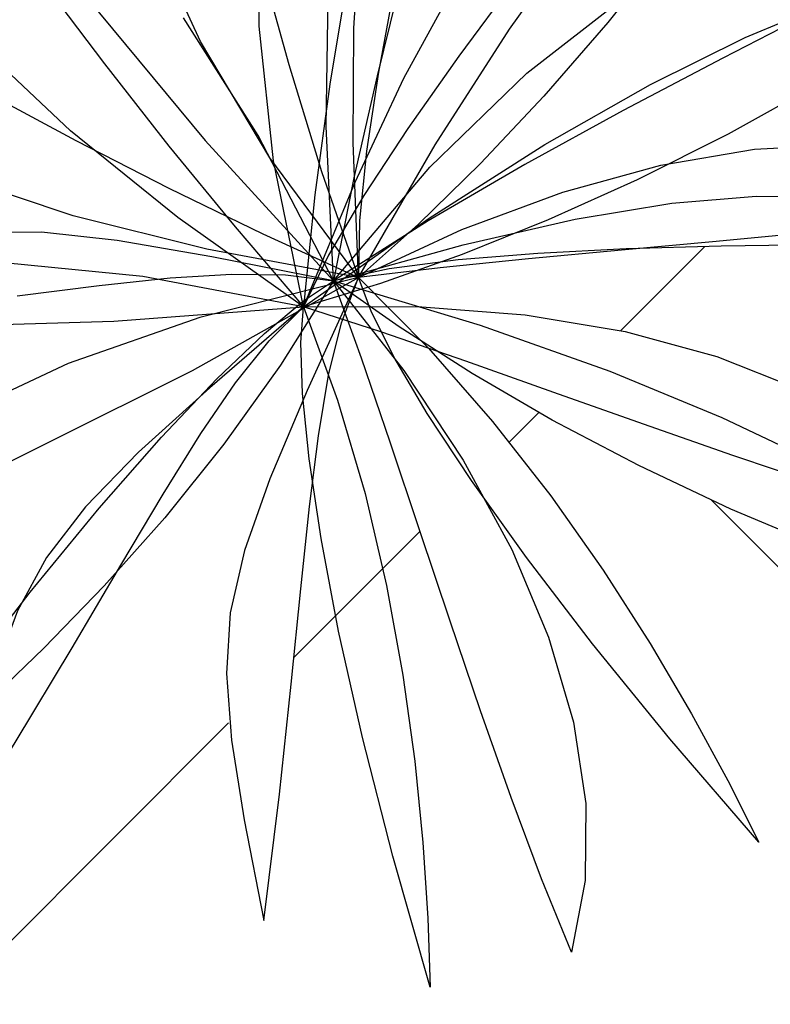
# Model space of a CAD drawing. Units: inches. Extents: x 3590 to 5167, y 65 to 1917.
# Tile 31 of 100: x 4947.17 to 4960.64, y 1339.27 to 1356.94. Entities that reach past the tile are written whole.
import ezdxf

# ---------------------------------------------------------------- set-up
doc = ezdxf.new("R2010")
doc.units = ezdxf.units.IN
doc.layers.add('A-FLOR-PATT', color=8, linetype='Continuous', lineweight=13)
doc.layers.add('L-PLNT', color=94, linetype='Continuous', lineweight=18)
doc.layers.add('DIENHOA', color=3, linetype='Continuous')

# ---------------------------------------------------------------- blocks, each defined once
blk = doc.blocks.new('Cay03_mb')
at = {"layer": 'DIENHOA'}
for p, q in [((-240.22, 277.83), (-88.39, 94.86)), ((55.75, 216.28), (37.33, 142.09)), ((0.21, 104.88), (1.62, 205.66)), ((146.96, 144.09), (218.51, 199.79)), ((363.69, 192.89), (290.19, 154.87)), ((-49.64, 98.45), (-104.15, 184.39)), ((290.19, 154.87), (217.38, 116.61)), ((75.94, 75.22), (146.96, 144.09)), ((37.33, 142.09), (20.49, 67.57)), ((217.38, 116.61), (145.48, 77.28)), ((5.39, -7.78), (0.21, 104.88)), ((-88.39, 94.86), (5.39, -7.78)), ((5.39, -7.78), (-49.64, 98.45)), ((5.39, -7.78), (75.94, 75.22)), ((145.48, 77.28), (74.74, 36.09)), ((20.49, 67.57), (5.39, -7.78)), ((252.97, 48.94), (314.63, 54.14)), ((314.63, 54.14), (369.18, 53.28)), ((182.2, 37.2), (252.97, 48.94)), ((74.74, 36.09), (5.39, -7.78)), ((100.34, 18.45), (182.2, 37.2)), ((-207.96, 27.76), (-254.73, 27.37)), ((-152.72, 21.72), (-207.96, 27.76)), ((-83.45, 9.72), (-152.72, 21.72)), ((5.39, -7.78), (100.34, 18.45)), ((219.62, 15.45), (154.97, 12.22)), ((289.03, 17.44), (219.62, 15.45)), ((361.61, 18.5), (289.03, 17.44)), ((5.39, -7.78), (-83.45, 9.72)), ((96.66, 7.47), (46.27, 0.9)), ((154.97, 12.22), (96.66, 7.47)), ((46.27, 0.9), (5.39, -7.78)), ((-165.8, -11.26), (-113.95, -5.74)), ((-113.95, -5.74), (-69, -2.91)), ((-69, -2.91), (-29.65, -3.38)), ((-29.65, -3.38), (5.39, -7.78)), ((-225.83, -18.85), (-165.8, -11.26)), ((5.39, -7.78), (-33.18, -69.47)), ((-16.51, -22.43), (5.39, -7.78)), ((5.39, -7.78), (56.83, -73.35)), ((25.88, -64.38), (5.39, -7.78)), ((5.39, -7.78), (112.81, -40.3)), ((53.47, -41.58), (5.39, -7.78)), ((-45.06, -46.34), (-16.51, -22.43)), ((106.98, -75.69), (53.47, -41.58)), ((112.81, -40.3), (207.46, -73.81)), ((-79.78, -79.55), (-45.06, -46.34)), ((47.05, -125.9), (25.88, -64.38)), ((-33.18, -69.47), (-74.57, -127.29)), ((56.83, -73.35), (100.42, -139.07)), ((165.52, -109.6), (106.98, -75.69)), ((207.46, -73.81), (289.55, -107.64)), ((-120.2, -122.13), (-79.78, -79.55)), ((289.55, -107.64), (359.29, -141.1)), ((228.67, -142.77), (165.52, -109.6)), ((-165.86, -174.12), (-120.2, -122.13)), ((-74.57, -127.29), (-117.85, -181.14)), ((68.74, -190.55), (47.05, -125.9)), ((100.42, -139.07), (135.85, -204.28)), ((296, -174.69), (228.67, -142.77)), ((-216.28, -235.58), (-165.86, -174.12)), ((367.1, -204.83), (296, -174.69)), ((-117.85, -181.14), (-162.07, -230.91)), ((90.79, -256.57), (68.74, -190.55)), ((135.85, -204.28), (162.8, -268.28)), ((-270.99, -306.55), (-216.28, -235.58)), ((-162.07, -230.91), (-206.29, -276.49)), ((113.06, -322.16), (90.79, -256.57)), ((162.8, -268.28), (180.96, -330.4)), ((-206.29, -276.49), (-249.56, -317.79)), ((135.38, -385.56), (113.06, -322.16)), ((180.96, -330.4), (190.01, -389.96)), ((157.6, -444.99), (135.38, -385.56)), ((190.01, -389.96), (189.65, -446.27)), ((179.55, -498.66), (157.6, -444.99)), ((189.65, -446.27), (179.55, -498.66))]:
    blk.add_line(p, q, dxfattribs=at)
for points in [[(23.69, -5.44), (-41, 82.2), (-91.83, 167.08), (-129.72, 249.45), (-155.55, 329.59), (-170.25, 407.76), (-174.71, 484.23), (-169.84, 559.26), (-156.54, 633.12)], [(-156.54, 633.12), (-132.46, 551.33), (-110.51, 470.02), (-89.84, 389.22), (-69.62, 308.98), (-48.99, 229.35), (-27.13, 150.38), (-3.18, 72.1), (23.69, -5.44)], [(-16.39, -26.73), (-38.34, 79.96), (-48.88, 178.33), (-48.7, 269), (-38.53, 352.58), (-19.08, 429.71), (8.95, 500.99), (44.86, 567.06), (87.92, 628.52)], [(87.92, 628.52), (75.46, 544.18), (61.27, 461.15), (46.13, 379.14), (30.83, 297.82), (16.14, 216.89), (2.85, 136.03), (-8.25, 54.92), (-16.39, -26.73)], [(23.69, -5.44), (19.84, 92.99), (20.28, 176.97), (25.02, 248.55), (34.03, 309.77), (47.33, 362.68), (64.91, 409.31), (86.75, 451.72), (112.87, 491.95)], [(112.87, 491.95), (95.99, 419.69), (79.46, 347.37), (63.92, 276.46), (50.01, 208.43), (38.38, 144.75), (29.69, 86.9), (24.57, 36.35), (23.69, -5.44)], [(-395.6, 473.65), (-347.51, 405.62), (-300.58, 339.5), (-254.33, 275.13), (-208.27, 212.32), (-161.92, 150.91), (-114.81, 90.72), (-66.46, 31.56), (-16.39, -26.73)], [(-16.39, -26.73), (-108.35, 38.55), (-186.88, 101.73), (-252.35, 163.45), (-305.09, 224.39), (-345.44, 285.22), (-373.75, 346.59), (-390.35, 409.18), (-395.6, 473.65)], [(384.28, 437.45), (342.25, 367.83), (298.14, 301.71), (252.56, 239.37), (206.11, 181.11), (159.39, 127.21), (113.01, 77.96), (67.57, 33.64), (23.69, -5.44)], [(23.69, -5.44), (79.88, 91.71), (134.12, 176.21), (185.81, 248.4), (234.31, 308.65), (279.02, 357.33), (319.33, 394.78), (354.62, 421.37), (384.28, 437.45)], [(273.24, 387.35), (227.6, 328.83), (182.25, 270.12), (138.39, 212.28), (97.23, 156.36), (59.96, 103.43), (27.8, 54.57), (1.94, 10.82), (-16.39, -26.73)], [(-16.39, -26.73), (21.41, 64.22), (57.05, 140.27), (91.37, 203.26), (125.24, 255.05), (159.51, 297.5), (195.03, 332.46), (232.65, 361.79), (273.24, 387.35)], [(-530.47, 289.69), (-458.27, 248.1), (-387.93, 207.77), (-318.94, 168.75), (-250.78, 131.06), (-182.94, 94.76), (-114.93, 59.88), (-46.22, 26.47), (23.69, -5.44)], [(23.69, -5.44), (-87.17, 15.25), (-184.97, 39.64), (-270.29, 68.2), (-343.73, 101.4), (-405.88, 139.68), (-457.33, 183.51), (-498.66, 233.36), (-530.47, 289.69)], [(496.74, 224.01), (429.38, 178.44), (361.6, 136.93), (294.07, 99.46), (227.46, 66.07), (162.44, 36.74), (99.68, 11.49), (39.84, -9.67), (-16.39, -26.73)], [(-16.39, -26.73), (75.38, 37.88), (160.06, 91.82), (237.27, 135.67), (306.57, 170.01), (367.58, 195.44), (419.88, 212.52), (463.07, 221.85), (496.74, 224.01)], [(23.69, -5.44), (99.27, 29.67), (173.22, 57.09), (244.79, 76.69), (313.26, 88.31), (377.88, 91.81), (437.93, 87.02), (492.67, 73.8), (541.37, 52)], [(541.37, 52), (484.11, 42.89), (421.18, 34.83), (354.36, 27.58), (285.41, 20.89), (216.1, 14.49), (148.2, 8.14), (83.47, 1.58), (23.69, -5.44)], [(-16.39, -26.73), (-133.98, -4.68), (-235.26, 5.29), (-321.98, 4.67), (-395.89, -5.03), (-458.73, -22.31), (-512.26, -45.67), (-558.22, -73.63), (-598.36, -104.66)], [(-471.89, -320.34), (-310.46, -179.32), (-97.66, -73.3), (23.69, -5.44)], [(23.69, -5.44), (-92.3, -34.76), (-188.42, -68.2), (-266.88, -105.14), (-329.9, -144.95), (-379.7, -187), (-418.48, -230.67), (-448.47, -275.32), (-471.89, -320.34)], [(23.69, -5.44), (-13.63, -87.94), (-41.14, -152.63), (-59.64, -205.04), (-69.94, -250.66), (-72.84, -295), (-69.17, -343.58), (-59.73, -401.89), (-45.32, -475.45)], [(-45.32, -475.45), (-34.09, -383.24), (-25.4, -302.82), (-18.34, -233.08), (-12.02, -172.9), (-5.55, -121.16), (1.96, -76.75), (11.41, -38.55), (23.69, -5.44)], [(316.49, -418.14), (251.44, -342.76), (194.84, -273.28), (146.52, -210.16), (106.33, -153.83), (74.11, -104.75), (49.71, -63.36), (32.95, -30.11), (23.69, -5.44)], [(23.69, -5.44), (74.94, -57.08), (121.78, -110.58), (164.32, -165.02), (202.67, -219.43), (236.95, -272.89), (267.27, -324.46), (293.75, -373.19), (316.49, -418.14)], [(-598.36, -104.66), (-392.67, -44.38), (-155.01, -37.42), (-16.39, -26.73)], [(-276.22, -424.43), (-227.35, -345.43), (-185.71, -276.08), (-150.05, -215.74), (-119.06, -163.76), (-91.49, -119.51), (-66.04, -82.35), (-41.43, -51.64), (-16.39, -26.73)], [(-16.39, -26.73), (-84.88, -85.96), (-136.99, -133.15), (-175.77, -172.96), (-204.26, -210.05), (-225.5, -249.08), (-242.55, -294.71), (-258.44, -351.61), (-276.22, -424.43)], [(76.25, -524.2), (48.83, -428.48), (26.6, -341.67), (9.22, -264.1), (-3.63, -196.11), (-12.28, -138.04), (-17.07, -90.23), (-18.33, -53.01), (-16.39, -26.73)], [(-16.39, -26.73), (66.95, -26.58), (145.58, -32.71), (218.77, -44.94), (285.79, -63.12), (345.92, -87.06), (398.42, -116.6), (442.57, -151.57), (477.63, -191.79)], [(477.63, -191.79), (421.82, -176.03), (361.32, -156.94), (297.62, -135.49), (232.22, -112.64), (166.63, -89.37), (102.33, -66.65), (40.82, -45.45), (-16.39, -26.73)], [(-16.39, -26.73), (8.47, -95.11), (28.54, -163.33), (44.32, -230.59), (56.3, -296.08), (64.99, -358.99), (70.88, -418.52), (74.46, -473.86), (76.25, -524.2)]]:
    blk.add_lwpolyline(points, dxfattribs=at)

msp = doc.modelspace()

# ---------------------------------------------------------------- hatches: boundary and pattern name
at = {"layer": 'A-FLOR-PATT', "transparency": 33554687}
h = msp.add_hatch(dxfattribs=at)
h.set_pattern_fill('AR-HBONE', color=256, scale=0.2)
h.set_pattern_definition([(45, (-588.972, 0), (0, 28.73682), [60.96, -20.32]), (135, (-574.604, 14.368), (3e-15, 28.73682), [60.96, -20.32])])
h.paths.add_polyline_path([(5071.274, 1796.999), (4933.274, 1796.999), (4933.274, 1753.999), (4962.774, 1753.999, -0.414214), (4928.774, 1719.999), (4933.274, 1718.999), (4933.274, 1334.999), (5071.274, 1334.999)])
h.paths.add_polyline_path([(4951.78, 1521.077), (4951.715, 1521.04), (4951.563, 1520.895)], flags=16)
h.paths.add_polyline_path([(4952.267, 1521.376), (4952.198, 1521.371), (4952.198, 1521.356)], flags=0)
h.paths.add_polyline_path([(4967.051, 1529.728), (4965.231, 1528.694), (4963.411, 1527.714), (4961.756, 1526.851), (4963.589, 1527.449), (4964.036, 1527.478), (4962.975, 1527.249), (4961.76, 1526.852), (4959.792, 1525.834), (4958.005, 1524.895), (4956.24, 1523.93), (4954.504, 1522.919), (4954.129, 1522.682), (4953.361, 1521.997), (4953.366, 1521.998), (4953.605, 1522.064), (4955.106, 1522.761), (4956.921, 1523.434), (4958.678, 1523.915), (4960.358, 1524.2), (4961.945, 1524.286), (4964.171, 1524.108), (4965.958, 1523.309), (4963.863, 1522.976), (4965.187, 1522.499), (4963.366, 1522.497), (4961.545, 1522.487), (4959.764, 1522.461), (4958.304, 1522.419), (4957.974, 1522.388), (4956.307, 1522.232), (4954.718, 1522.071), (4953.251, 1521.899), (4953.525, 1521.623), (4954.331, 1521.379), (4956.243, 1521.23), (4958.039, 1520.93), (4959.684, 1520.483), (4961.16, 1519.896), (4963.107, 1518.8), (4964.393, 1517.325), (4962.973, 1517.726), (4964.558, 1516.661), (4965.407, 1515.708), (4963.507, 1516.322), (4961.68, 1517.005), (4959.935, 1517.745), (4958.282, 1518.528), (4956.732, 1519.343), (4955.295, 1520.175), (4954.672, 1520.572), (4954.513, 1520.627), (4955.658, 1519.318), (4956.703, 1517.982), (4957.644, 1516.647), (4958.485, 1515.334), (4959.55, 1513.524), (4960.438, 1511.769), (4958.841, 1513.62), (4957.452, 1515.325), (4955.819, 1517.459), (4956.665, 1515.448), (4957.111, 1513.923), (4957.447, 1511.714), (4957.076, 1509.793), (4956.538, 1511.11), (4955.992, 1512.569), (4955.444, 1514.125), (4954.898, 1515.735), (4954.357, 1517.356), (4953.824, 1518.943), (4953.305, 1520.452), (4953.065, 1521.116), (4952.971, 1521.146), (4952.949, 1521.086), (4952.73, 1520.199), (4953.37, 1518.024), (4953.757, 1516.373), (4954.051, 1514.765), (4954.264, 1513.221), (4954.471, 1511.131), (4954.497, 1510.402), (4954.409, 1511.76), (4954.264, 1513.221), (4954.051, 1514.765), (4953.757, 1516.373), (4953.37, 1518.024), (4952.877, 1519.698), (4952.716, 1520.141), (4952.533, 1519.059), (4952.374, 1517.789), (4952.219, 1516.312), (4952.046, 1514.6), (4951.833, 1512.626), (4951.557, 1510.363), (4951.203, 1512.168), (4950.852, 1514.339), (4950.985, 1516.376), (4951.66, 1518.286), (4952.593, 1520.481), (4952.357, 1521.13), (4951.855, 1520.328), (4950.839, 1518.908), (4949.777, 1517.587), (4948.916, 1516.617), (4948.111, 1515.256), (4947.089, 1513.554), (4945.889, 1511.615), (4946.326, 1513.402), (4946.562, 1514.249), (4945.528, 1513.327), (4944.581, 1512.531), (4946.018, 1514.508), (4947.204, 1516.048), (4947.893, 1517.313), (4949.307, 1518.764), (4950.414, 1519.767), (4950.451, 1519.806), (4952.267, 1521.376), (4951.645, 1521.493), (4950.404, 1521.18), (4948.044, 1520.359), (4946.119, 1519.452), (4944.572, 1518.475), (4943.35, 1517.443), (4941.997, 1515.92), (4941.661, 1515.275), (4942.813, 1516.99), (4944.572, 1518.475), (4946.119, 1519.452), (4948.044, 1520.359), (4950.404, 1521.18), (4951.645, 1521.493), (4949.647, 1521.868), (4948.6, 1521.756), (4947.126, 1521.57), (4945.42, 1521.348), (4943.45, 1521.105), (4941.183, 1520.856), (4942.86, 1521.613), (4943.873, 1522.03), (4942.952, 1521.909), (4941.41, 1521.485), (4939.543, 1520.67), (4938.968, 1520.226), (4940.733, 1521.299), (4942.952, 1521.909), (4943.702, 1522.008), (4945.894, 1522.7), (4947.565, 1522.714), (4948.921, 1522.566), (4951.131, 1522.183), (4950.971, 1522.297), (4948.129, 1523.006), (4946.035, 1523.707), (4944.232, 1524.521), (4942.707, 1525.461), (4941.444, 1526.537), (4940.43, 1527.761), (4939.649, 1529.143), (4941.421, 1528.122), (4943.147, 1527.132), (4944.841, 1526.175), (4946.514, 1525.25), (4948.179, 1524.359), (4948.365, 1524.263), (4946.475, 1526.045), (4945.181, 1527.54), (4944.19, 1529.033), (4943.496, 1530.54), (4943.278, 1531.36), (4942.498, 1531.919), (4943.114, 1531.762), (4942.959, 1533.659), (4944.14, 1531.989), (4944.612, 1531.323), (4946.202, 1530.463), (4947.486, 1529.509), (4948.79, 1528.226), (4950.368, 1526.237), (4949.485, 1528.155), (4948.851, 1530.123), (4948.491, 1532.041), (4948.381, 1533.918), (4948.501, 1535.76), (4948.827, 1537.573), (4949.418, 1535.565), (4949.957, 1533.569), (4950.464, 1531.586), (4950.961, 1529.617), (4951.391, 1527.954), (4951.724, 1530.687), (4952.201, 1532.58), (4952.889, 1534.33), (4953.77, 1535.951), (4954.827, 1537.46), (4954.521, 1535.39), (4954.273, 1533.937), (4955.58, 1535.663), (4956.748, 1536.739), (4956.159, 1534.78), (4955.589, 1532.873), (4955.043, 1531.006), (4954.525, 1529.166), (4954.038, 1527.341), (4953.638, 1525.733), (4953.611, 1525.586), (4953.398, 1524.166), (4953.382, 1524.009), (4954.07, 1525.476), (4954.912, 1527.022), (4956.136, 1528.894), (4957.847, 1530.577), (4959.376, 1531.54), (4958.256, 1530.104), (4957.143, 1528.663), (4956.066, 1527.243), (4955.056, 1525.871), (4954.141, 1524.571), (4953.352, 1523.372), (4953.311, 1523.303), (4953.273, 1522.925), (4953.261, 1522.382), (4954.103, 1523.373), (4954.63, 1524.284), (4955.961, 1526.358), (4957.23, 1528.13), (4958.421, 1529.609), (4960.037, 1531.368), (4961.374, 1532.375), (4962.101, 1532.77), (4961.07, 1531.061), (4959.987, 1529.438), (4958.869, 1527.908), (4958.15, 1527.007), (4959.803, 1528.003), (4961.589, 1528.793), (4963.391, 1529.328), (4965.211, 1529.632)], flags=16)
h.paths.add_polyline_path([(4962.944, 1523.182), (4961.107, 1523.422), (4960.392, 1523.362), (4962.35, 1523.331)], flags=0)
h.paths.add_polyline_path([(5049.541, 1584.551), (5049.476, 1584.515), (5049.325, 1584.37)], flags=16)
h.paths.add_polyline_path([(5050.028, 1584.851), (5049.959, 1584.845), (5049.959, 1584.83)], flags=0)
h.paths.add_polyline_path([(5042.333, 1581.949), (5043.88, 1582.926), (5045.806, 1583.833), (5048.165, 1584.654), (5049.406, 1584.967), (5047.408, 1585.342), (5046.361, 1585.231), (5044.888, 1585.044), (5043.181, 1584.822), (5041.211, 1584.579), (5038.944, 1584.33), (5040.622, 1585.087), (5041.634, 1585.504), (5040.713, 1585.383), (5039.171, 1584.959), (5037.304, 1584.144), (5036.729, 1583.7), (5038.494, 1584.773), (5040.713, 1585.383), (5041.463, 1585.482), (5043.655, 1586.174), (5045.326, 1586.188), (5046.682, 1586.04), (5048.893, 1585.657), (5048.732, 1585.771), (5045.891, 1586.48), (5043.796, 1587.181), (5041.994, 1587.996), (5040.468, 1588.935), (5039.205, 1590.011), (5038.191, 1591.235), (5037.41, 1592.617), (5039.182, 1591.596), (5040.909, 1590.607), (5042.602, 1589.649), (5044.275, 1588.724), (5045.94, 1587.833), (5046.126, 1587.738), (5044.237, 1589.519), (5042.942, 1591.015), (5041.952, 1592.508), (5041.257, 1594.014), (5041.039, 1594.834), (5040.26, 1595.393), (5040.875, 1595.237), (5040.721, 1597.133), (5041.901, 1595.463), (5042.373, 1594.798), (5043.963, 1593.938), (5045.247, 1592.983), (5046.552, 1591.701), (5048.129, 1589.712), (5047.247, 1591.63), (5046.613, 1593.597), (5046.252, 1595.515), (5046.142, 1597.392), (5046.262, 1599.234), (5046.588, 1601.047), (5047.179, 1599.039), (5047.718, 1597.043), (5048.225, 1595.06), (5048.722, 1593.091), (5049.152, 1591.429), (5049.485, 1594.161), (5049.962, 1596.054), (5050.65, 1597.804), (5051.532, 1599.425), (5052.589, 1600.934), (5052.283, 1598.864), (5052.034, 1597.411), (5053.341, 1599.137), (5054.509, 1600.213), (5053.92, 1598.254), (5053.35, 1596.348), (5052.805, 1594.48), (5052.286, 1592.64), (5051.799, 1590.815), (5051.4, 1589.207), (5051.373, 1589.06), (5051.159, 1587.64), (5051.143, 1587.483), (5051.831, 1588.95), (5052.673, 1590.496), (5053.898, 1592.368), (5055.608, 1594.051), (5057.137, 1595.014), (5056.017, 1593.578), (5054.904, 1592.137), (5053.828, 1590.717), (5052.817, 1589.345), (5051.902, 1588.046), (5051.113, 1586.846), (5051.072, 1586.777), (5051.034, 1586.399), (5051.022, 1585.856), (5051.864, 1586.847), (5052.391, 1587.758), (5053.723, 1589.832), (5054.991, 1591.604), (5056.182, 1593.083), (5057.798, 1594.842), (5059.135, 1595.849), (5059.863, 1596.244), (5058.831, 1594.535), (5057.749, 1592.912), (5056.63, 1591.382), (5055.912, 1590.482), (5057.564, 1591.477), (5059.35, 1592.267), (5061.152, 1592.802), (5062.972, 1593.106), (5064.812, 1593.203), (5062.992, 1592.169), (5061.172, 1591.188), (5059.518, 1590.325), (5061.35, 1590.924), (5061.797, 1590.952), (5060.737, 1590.723), (5059.521, 1590.326), (5057.553, 1589.308), (5055.766, 1588.369), (5054.002, 1587.404), (5052.265, 1586.393), (5051.891, 1586.156), (5051.122, 1585.471), (5051.127, 1585.472), (5051.366, 1585.538), (5052.867, 1586.235), (5054.682, 1586.908), (5056.439, 1587.389), (5058.12, 1587.675), (5059.706, 1587.76), (5061.933, 1587.583), (5063.719, 1586.783), (5061.624, 1586.45), (5062.949, 1585.973), (5061.127, 1585.971), (5059.307, 1585.961), (5057.525, 1585.935), (5056.065, 1585.893), (5055.735, 1585.862), (5054.068, 1585.707), (5052.479, 1585.546), (5051.012, 1585.373), (5051.286, 1585.097), (5052.092, 1584.853), (5054.004, 1584.704), (5055.8, 1584.404), (5057.446, 1583.958), (5058.921, 1583.37), (5060.868, 1582.274), (5062.154, 1580.799), (5060.734, 1581.2), (5062.32, 1580.135), (5063.168, 1579.182), (5061.269, 1579.796), (5059.441, 1580.479), (5057.696, 1581.219), (5056.043, 1582.003), (5054.493, 1582.817), (5053.057, 1583.649), (5052.433, 1584.047), (5052.274, 1584.101), (5053.42, 1582.793), (5054.464, 1581.457), (5055.405, 1580.121), (5056.247, 1578.809), (5057.311, 1576.998), (5058.199, 1575.244), (5056.602, 1577.094), (5055.213, 1578.799), (5053.58, 1580.933), (5054.427, 1578.922), (5054.872, 1577.397), (5055.208, 1575.189), (5054.838, 1573.267), (5054.299, 1574.584), (5053.754, 1576.043), (5053.206, 1577.599), (5052.659, 1579.209), (5052.118, 1580.83), (5051.585, 1582.417), (5051.066, 1583.927), (5050.826, 1584.59), (5050.733, 1584.62), (5050.711, 1584.561), (5050.491, 1583.673), (5051.131, 1581.498), (5051.518, 1579.847), (5051.813, 1578.24), (5052.026, 1576.695), (5052.233, 1574.605), (5052.258, 1573.876), (5052.17, 1575.234), (5052.026, 1576.695), (5051.813, 1578.24), (5051.518, 1579.847), (5051.131, 1581.498), (5050.638, 1583.172), (5050.477, 1583.615), (5050.294, 1582.533), (5050.136, 1581.263), (5049.981, 1579.786), (5049.807, 1578.074), (5049.594, 1576.1), (5049.318, 1573.837), (5048.965, 1575.642), (5048.613, 1577.813), (5048.747, 1579.85), (5049.421, 1581.76), (5050.354, 1583.955), (5050.118, 1584.604), (5049.616, 1583.802), (5048.6, 1582.382), (5047.538, 1581.061), (5046.677, 1580.091), (5045.872, 1578.73), (5044.85, 1577.028), (5043.651, 1575.089), (5044.087, 1576.877), (5044.324, 1577.723), (5043.289, 1576.801), (5042.342, 1576.005), (5043.779, 1577.982), (5044.966, 1579.522), (5045.655, 1580.787), (5047.068, 1582.239), (5048.175, 1583.241), (5048.213, 1583.28), (5050.028, 1584.851), (5049.406, 1584.967), (5048.165, 1584.654), (5045.806, 1583.833), (5043.88, 1582.926), (5042.333, 1581.949), (5041.111, 1580.917), (5039.758, 1579.394), (5039.423, 1578.749), (5040.575, 1580.464)], flags=16)
h.paths.add_polyline_path([(4954.799, 1533.12), (4954.262, 1532.079), (4953.831, 1530.935), (4953.505, 1529.636), (4953.283, 1528.133), (4953.167, 1526.376), (4953.156, 1524.315), (4953.277, 1521.236), (4952.802, 1521.842), (4951.557, 1521.998), (4950.976, 1521.961), (4952.661, 1521.941), (4952.802, 1521.842), (4953.152, 1523.593), (4953.167, 1526.376), (4953.283, 1528.133), (4953.609, 1530.346), (4954.456, 1532.592)], flags=0)
h.paths.add_polyline_path([(5050.563, 1585.316), (5049.318, 1585.472), (5048.737, 1585.435), (5050.422, 1585.415), (5050.563, 1585.316), (5050.914, 1587.067), (5050.928, 1589.851), (5051.045, 1591.607), (5051.371, 1593.82), (5052.217, 1596.066), (5052.56, 1596.594), (5052.024, 1595.554), (5051.592, 1594.409), (5051.266, 1593.11), (5051.045, 1591.607), (5050.928, 1589.851), (5050.918, 1587.789), (5051.038, 1584.71)], flags=0)
h.paths.add_polyline_path([(5058.153, 1586.836), (5060.111, 1586.805), (5060.705, 1586.656), (5058.868, 1586.896)], flags=0)
h.paths.add_polyline_path([(5049.541, 1430.936), (5049.476, 1430.9), (5049.325, 1430.755)], flags=16)
h.paths.add_polyline_path([(5050.028, 1431.236), (5049.959, 1431.231), (5049.959, 1431.215)], flags=0)
h.paths.add_polyline_path([(5046.588, 1447.432), (5047.179, 1445.425), (5047.718, 1443.429), (5048.225, 1441.446), (5048.722, 1439.476), (5049.152, 1437.814), (5049.485, 1440.546), (5049.962, 1442.439), (5050.65, 1444.189), (5051.532, 1445.811), (5052.589, 1447.319), (5052.283, 1445.249), (5052.034, 1443.796), (5053.341, 1445.522), (5054.509, 1446.598), (5053.92, 1444.64), (5053.35, 1442.733), (5052.805, 1440.865), (5052.286, 1439.025), (5051.799, 1437.201), (5051.4, 1435.592), (5051.373, 1435.445), (5051.159, 1434.025), (5051.143, 1433.868), (5051.831, 1435.335), (5052.673, 1436.881), (5053.898, 1438.753), (5055.608, 1440.436), (5057.137, 1441.4), (5056.017, 1439.963), (5054.904, 1438.522), (5053.828, 1437.102), (5052.817, 1435.73), (5051.902, 1434.431), (5051.113, 1433.231), (5051.072, 1433.162), (5051.034, 1432.784), (5051.022, 1432.242), (5051.864, 1433.232), (5052.391, 1434.143), (5053.723, 1436.217), (5054.991, 1437.989), (5056.182, 1439.468), (5057.798, 1441.227), (5059.135, 1442.235), (5059.863, 1442.629), (5058.831, 1440.921), (5057.749, 1439.298), (5056.63, 1437.767), (5055.912, 1436.867), (5057.564, 1437.863), (5059.35, 1438.652), (5061.152, 1439.187), (5062.972, 1439.491), (5064.812, 1439.588), (5062.992, 1438.554), (5061.172, 1437.573), (5059.518, 1436.71), (5061.35, 1437.309), (5061.797, 1437.337), (5060.737, 1437.108), (5059.521, 1436.711), (5057.553, 1435.693), (5055.766, 1434.754), (5054.002, 1433.789), (5052.265, 1432.778), (5051.891, 1432.541), (5051.122, 1431.856), (5051.127, 1431.857), (5051.366, 1431.923), (5052.867, 1432.62), (5054.682, 1433.293), (5056.439, 1433.775), (5058.12, 1434.06), (5059.706, 1434.145), (5061.933, 1433.968), (5063.719, 1433.168), (5061.624, 1432.835), (5062.949, 1432.358), (5061.127, 1432.357), (5059.307, 1432.346), (5057.525, 1432.32), (5056.065, 1432.278), (5055.735, 1432.248), (5054.068, 1432.092), (5052.479, 1431.931), (5051.012, 1431.759), (5051.286, 1431.482), (5052.092, 1431.238), (5054.004, 1431.089), (5055.8, 1430.789), (5057.446, 1430.343), (5058.921, 1429.755), (5060.868, 1428.66), (5062.154, 1427.185), (5060.734, 1427.585), (5062.32, 1426.52), (5063.168, 1425.567), (5061.269, 1426.181), (5059.441, 1426.865), (5057.696, 1427.604), (5056.043, 1428.388), (5054.493, 1429.202), (5053.057, 1430.034), (5052.433, 1430.432), (5052.274, 1430.487), (5053.42, 1429.178), (5054.464, 1427.842), (5055.405, 1426.506), (5056.247, 1425.194), (5057.311, 1423.383), (5058.199, 1421.629), (5056.602, 1423.479), (5055.213, 1425.184), (5053.58, 1427.318), (5054.427, 1425.307), (5054.872, 1423.782), (5055.208, 1421.574), (5054.838, 1419.652), (5054.299, 1420.97), (5053.754, 1422.428), (5053.206, 1423.984), (5052.659, 1425.595), (5052.118, 1427.215), (5051.585, 1428.802), (5051.066, 1430.312), (5050.826, 1430.975), (5050.733, 1431.005), (5050.711, 1430.946), (5050.491, 1430.058), (5051.131, 1427.883), (5051.518, 1426.232), (5051.813, 1424.625), (5052.026, 1423.081), (5052.233, 1420.991), (5052.258, 1420.261), (5052.17, 1421.619), (5052.026, 1423.081), (5051.813, 1424.625), (5051.518, 1426.232), (5051.131, 1427.883), (5050.638, 1429.558), (5050.477, 1430.001), (5050.294, 1428.918), (5050.136, 1427.648), (5049.981, 1426.171), (5049.807, 1424.459), (5049.594, 1422.485), (5049.318, 1420.222), (5048.965, 1422.028), (5048.613, 1424.199), (5048.747, 1426.235), (5049.421, 1428.146), (5050.354, 1430.34), (5050.118, 1430.989), (5049.616, 1430.187), (5048.6, 1428.768), (5047.538, 1427.446), (5046.677, 1426.477), (5045.872, 1425.116), (5044.85, 1423.413), (5043.651, 1421.474), (5044.087, 1423.262), (5044.324, 1424.109), (5043.289, 1423.186), (5042.342, 1422.391), (5043.779, 1424.368), (5044.966, 1425.907), (5045.655, 1427.173), (5047.068, 1428.624), (5048.175, 1429.627), (5048.213, 1429.666), (5050.028, 1431.236), (5049.406, 1431.353), (5048.165, 1431.039), (5045.806, 1430.218), (5043.88, 1429.311), (5042.333, 1428.334), (5041.111, 1427.302), (5039.758, 1425.779), (5039.423, 1425.134), (5040.575, 1426.849), (5042.333, 1428.334), (5043.88, 1429.311), (5045.806, 1430.218), (5048.165, 1431.039), (5049.406, 1431.353), (5047.408, 1431.727), (5046.361, 1431.616), (5044.888, 1431.429), (5043.181, 1431.207), (5041.211, 1430.964), (5038.944, 1430.715), (5040.622, 1431.472), (5041.634, 1431.89), (5040.713, 1431.769), (5039.171, 1431.345), (5037.304, 1430.53), (5036.729, 1430.085), (5038.494, 1431.158), (5040.713, 1431.769), (5041.463, 1431.867), (5043.655, 1432.559), (5045.326, 1432.573), (5046.682, 1432.425), (5048.893, 1432.042), (5048.732, 1432.156), (5045.891, 1432.865), (5043.796, 1433.566), (5041.994, 1434.381), (5040.468, 1435.321), (5039.205, 1436.396), (5038.191, 1437.62), (5037.41, 1439.002), (5039.182, 1437.982), (5040.909, 1436.992), (5042.602, 1436.034), (5044.275, 1435.109), (5045.94, 1434.218), (5046.126, 1434.123), (5044.237, 1435.904), (5042.942, 1437.4), (5041.952, 1438.893), (5041.257, 1440.399), (5041.039, 1441.219), (5040.26, 1441.778), (5040.875, 1441.622), (5040.721, 1443.518), (5041.901, 1441.848), (5042.373, 1441.183), (5043.963, 1440.323), (5045.247, 1439.369), (5046.552, 1438.086), (5048.129, 1436.097), (5047.247, 1438.015), (5046.613, 1439.982), (5046.252, 1441.901), (5046.142, 1443.778), (5046.262, 1445.619)], flags=16)
h.paths.add_polyline_path([(5052.382, 1444.255), (5051.623, 1442.78), (5052.024, 1441.939), (5052.56, 1442.98)], flags=0)
h.paths.add_polyline_path([(5050.563, 1431.701), (5049.318, 1431.857), (5048.737, 1431.821), (5050.422, 1431.8)], flags=0)
h.paths.add_polyline_path([(5058.153, 1433.221), (5060.111, 1433.19), (5060.705, 1433.041), (5058.868, 1433.281)], flags=0)
h.paths.add_polyline_path([(5049.541, 1352.285), (5049.476, 1352.249), (5049.325, 1352.104)], flags=16)
h.paths.add_polyline_path([(5050.028, 1352.585), (5049.959, 1352.58), (5049.959, 1352.564)], flags=0)
h.paths.add_polyline_path([(5046.588, 1368.781), (5047.179, 1366.774), (5047.718, 1364.778), (5048.225, 1362.795), (5048.722, 1360.825), (5049.152, 1359.163), (5049.485, 1361.896), (5049.962, 1363.789), (5050.65, 1365.538), (5051.532, 1367.16), (5052.589, 1368.669), (5052.283, 1366.598), (5052.034, 1365.145), (5053.341, 1366.871), (5054.509, 1367.947), (5053.92, 1365.989), (5053.35, 1364.082), (5052.805, 1362.214), (5052.286, 1360.374), (5051.799, 1358.55), (5051.4, 1356.942), (5051.373, 1356.794), (5051.159, 1355.374), (5051.143, 1355.218), (5051.831, 1356.684), (5052.673, 1358.23), (5053.898, 1360.102), (5055.608, 1361.786), (5057.137, 1362.749), (5056.017, 1361.313), (5054.904, 1359.872), (5053.828, 1358.452), (5052.817, 1357.079), (5051.902, 1355.78), (5051.113, 1354.581), (5051.072, 1354.512), (5051.034, 1354.133), (5051.022, 1353.591), (5051.864, 1354.581), (5052.391, 1355.492), (5053.723, 1357.566), (5054.991, 1359.338), (5056.182, 1360.817), (5057.798, 1362.577), (5059.135, 1363.584), (5059.863, 1363.979), (5058.831, 1362.27), (5057.749, 1360.647), (5056.63, 1359.117), (5055.912, 1358.216), (5057.564, 1359.212), (5059.35, 1360.001), (5061.152, 1360.536), (5062.972, 1360.841), (5064.812, 1360.937), (5062.992, 1359.903), (5061.172, 1358.923), (5059.518, 1358.059), (5061.35, 1358.658), (5061.797, 1358.687), (5060.737, 1358.458), (5059.521, 1358.061), (5057.553, 1357.043), (5055.766, 1356.103), (5054.002, 1355.138), (5052.265, 1354.127), (5051.891, 1353.89), (5051.122, 1353.206), (5051.127, 1353.206), (5051.366, 1353.272), (5052.867, 1353.969), (5054.682, 1354.643), (5056.439, 1355.124), (5058.12, 1355.409), (5059.706, 1355.495), (5061.933, 1355.317), (5063.719, 1354.518), (5061.624, 1354.184), (5062.949, 1353.708), (5061.127, 1353.706), (5059.307, 1353.695), (5057.525, 1353.669), (5056.065, 1353.627), (5055.735, 1353.597), (5054.068, 1353.441), (5052.479, 1353.28), (5051.012, 1353.108), (5051.286, 1352.831), (5052.092, 1352.587), (5054.004, 1352.439), (5055.8, 1352.138), (5057.446, 1351.692), (5058.921, 1351.104), (5060.868, 1350.009), (5062.154, 1348.534), (5060.734, 1348.935), (5062.32, 1347.869), (5063.168, 1346.916), (5061.269, 1347.53), (5059.441, 1348.214), (5057.696, 1348.954), (5056.043, 1349.737), (5054.493, 1350.551), (5053.057, 1351.383), (5052.433, 1351.781), (5052.274, 1351.836), (5053.42, 1350.527), (5054.464, 1349.191), (5055.405, 1347.855), (5056.247, 1346.543), (5057.311, 1344.733), (5058.199, 1342.978), (5056.602, 1344.828), (5055.213, 1346.534), (5053.58, 1348.667), (5054.427, 1346.656), (5054.872, 1345.132), (5055.208, 1342.923), (5054.838, 1341.002), (5054.299, 1342.319), (5053.754, 1343.778), (5053.206, 1345.334), (5052.659, 1346.944), (5052.118, 1348.564), (5051.585, 1350.151), (5051.066, 1351.661), (5050.826, 1352.324), (5050.733, 1352.355), (5050.711, 1352.295), (5050.491, 1351.408), (5051.131, 1349.232), (5051.518, 1347.581), (5051.813, 1345.974), (5052.026, 1344.43), (5052.233, 1342.34), (5052.258, 1341.61), (5052.17, 1342.969), (5052.026, 1344.43), (5051.813, 1345.974), (5051.518, 1347.581), (5051.131, 1349.232), (5050.638, 1350.907), (5050.477, 1351.35), (5050.294, 1350.267), (5050.136, 1348.997), (5049.981, 1347.52), (5049.807, 1345.809), (5049.594, 1343.835), (5049.318, 1341.571), (5048.965, 1343.377), (5048.613, 1345.548), (5048.747, 1347.585), (5049.421, 1349.495), (5050.354, 1351.689), (5050.118, 1352.339), (5049.616, 1351.536), (5048.6, 1350.117), (5047.538, 1348.795), (5046.677, 1347.826), (5045.872, 1346.465), (5044.85, 1344.763), (5043.651, 1342.824), (5044.087, 1344.611), (5044.324, 1345.458), (5043.289, 1344.535), (5042.342, 1343.74), (5043.779, 1345.717), (5044.966, 1347.256), (5045.655, 1348.522), (5047.068, 1349.973), (5048.175, 1350.976), (5048.213, 1351.015), (5050.028, 1352.585), (5049.406, 1352.702), (5048.165, 1352.388), (5045.806, 1351.567), (5043.88, 1350.661), (5042.333, 1349.683), (5041.111, 1348.651), (5039.758, 1347.128), (5039.423, 1346.483), (5040.575, 1348.198), (5042.333, 1349.683), (5043.88, 1350.661), (5045.806, 1351.567), (5048.165, 1352.388), (5049.406, 1352.702), (5047.408, 1353.076), (5046.361, 1352.965), (5044.888, 1352.779), (5043.181, 1352.556), (5041.211, 1352.313), (5038.944, 1352.065), (5040.622, 1352.821), (5041.634, 1353.239), (5040.713, 1353.118), (5039.171, 1352.694), (5037.304, 1351.879), (5036.729, 1351.434), (5038.494, 1352.508), (5040.713, 1353.118), (5041.463, 1353.216), (5043.655, 1353.909), (5045.326, 1353.923), (5046.682, 1353.774), (5048.893, 1353.391), (5048.732, 1353.506), (5045.891, 1354.214), (5043.796, 1354.915), (5041.994, 1355.73), (5040.468, 1356.67), (5039.205, 1357.746), (5038.191, 1358.969), (5037.41, 1360.352), (5039.182, 1359.331), (5040.909, 1358.341), (5042.602, 1357.383), (5044.275, 1356.458), (5045.94, 1355.567), (5046.126, 1355.472), (5044.237, 1357.253), (5042.942, 1358.749), (5041.952, 1360.242), (5041.257, 1361.748), (5041.039, 1362.568), (5040.26, 1363.128), (5040.875, 1362.971), (5040.721, 1364.867), (5041.901, 1363.197), (5042.373, 1362.532), (5043.963, 1361.672), (5045.247, 1360.718), (5046.552, 1359.435), (5048.129, 1357.446), (5047.247, 1359.364), (5046.613, 1361.331), (5046.252, 1363.25), (5046.142, 1365.127), (5046.262, 1366.969)], flags=16)
h.paths.add_polyline_path([(5052.382, 1365.604), (5051.623, 1364.129), (5052.024, 1363.288), (5052.56, 1364.329)], flags=0)
h.paths.add_polyline_path([(4951.78, 1698.041), (4951.715, 1698.005), (4951.563, 1697.859)], flags=16)
h.paths.add_polyline_path([(4952.267, 1698.341), (4952.198, 1698.335), (4952.198, 1698.32)], flags=0)
h.paths.add_polyline_path([(4957.076, 1686.757), (4956.538, 1688.074), (4955.992, 1689.533), (4955.444, 1691.089), (4954.898, 1692.699), (4954.357, 1694.32), (4953.824, 1695.907), (4953.305, 1697.417), (4953.065, 1698.08), (4952.971, 1698.11), (4952.949, 1698.051), (4952.73, 1697.163), (4953.37, 1694.988), (4953.757, 1693.337), (4954.051, 1691.729), (4954.264, 1690.185), (4954.471, 1688.095), (4954.497, 1687.366), (4954.409, 1688.724), (4954.264, 1690.185), (4954.051, 1691.729), (4953.757, 1693.337), (4953.37, 1694.988), (4952.877, 1696.662), (4952.716, 1697.105), (4952.533, 1696.023), (4952.374, 1694.753), (4952.219, 1693.276), (4952.046, 1691.564), (4951.833, 1689.59), (4951.557, 1687.327), (4951.203, 1689.132), (4950.852, 1691.303), (4950.985, 1693.34), (4951.66, 1695.25), (4952.593, 1697.445), (4952.357, 1698.094), (4951.855, 1697.292), (4950.839, 1695.872), (4949.777, 1694.551), (4948.916, 1693.581), (4948.111, 1692.22), (4947.089, 1690.518), (4945.889, 1688.579), (4946.326, 1690.366), (4946.562, 1691.213), (4945.528, 1690.291), (4944.581, 1689.495), (4946.018, 1691.472), (4947.204, 1693.012), (4947.893, 1694.277), (4949.307, 1695.729), (4950.414, 1696.731), (4950.451, 1696.77), (4952.267, 1698.341), (4951.645, 1698.457), (4950.404, 1698.144), (4948.044, 1697.323), (4946.119, 1696.416), (4944.572, 1695.439), (4943.35, 1694.407), (4941.997, 1692.884), (4941.661, 1692.239), (4942.813, 1693.954), (4944.572, 1695.439), (4946.119, 1696.416), (4948.044, 1697.323), (4950.404, 1698.144), (4951.645, 1698.457), (4949.647, 1698.832), (4948.6, 1698.72), (4947.126, 1698.534), (4945.42, 1698.312), (4943.45, 1698.069), (4941.183, 1697.82), (4942.86, 1698.577), (4943.873, 1698.994), (4942.952, 1698.873), (4941.41, 1698.449), (4939.543, 1697.634), (4938.968, 1697.19), (4940.733, 1698.263), (4942.952, 1698.873), (4943.702, 1698.972), (4945.894, 1699.664), (4947.565, 1699.678), (4948.921, 1699.53), (4951.131, 1699.147), (4950.971, 1699.261), (4948.129, 1699.97), (4946.035, 1700.671), (4944.232, 1701.486), (4942.707, 1702.425), (4941.444, 1703.501), (4940.43, 1704.725), (4939.649, 1706.107), (4941.421, 1705.086), (4943.147, 1704.097), (4944.841, 1703.139), (4946.514, 1702.214), (4948.179, 1701.323), (4948.365, 1701.227), (4946.475, 1703.009), (4945.181, 1704.505), (4944.19, 1705.997), (4943.496, 1707.504), (4943.278, 1708.324), (4942.498, 1708.883), (4943.114, 1708.727), (4942.959, 1710.623), (4944.14, 1708.953), (4944.612, 1708.287), (4946.202, 1707.428), (4947.486, 1706.473), (4948.79, 1705.191), (4950.368, 1703.202), (4949.485, 1705.12), (4948.851, 1707.087), (4948.491, 1709.005), (4948.381, 1710.882), (4948.501, 1712.724), (4948.827, 1714.537), (4949.418, 1712.529), (4949.957, 1710.533), (4950.464, 1708.55), (4950.961, 1706.581), (4951.391, 1704.919), (4951.724, 1707.651), (4952.201, 1709.544), (4952.889, 1711.294), (4953.77, 1712.915), (4954.827, 1714.424), (4954.521, 1712.354), (4954.273, 1710.901), (4955.58, 1712.627), (4956.748, 1713.703), (4956.159, 1711.744), (4955.589, 1709.837), (4955.043, 1707.97), (4954.525, 1706.13), (4954.038, 1704.305), (4953.638, 1702.697), (4953.611, 1702.55), (4953.398, 1701.13), (4953.382, 1700.973), (4954.07, 1702.44), (4954.912, 1703.986), (4956.136, 1705.858), (4957.847, 1707.541), (4959.376, 1708.504), (4958.256, 1707.068), (4957.143, 1705.627), (4956.066, 1704.207), (4955.056, 1702.835), (4954.141, 1701.536), (4953.352, 1700.336), (4953.311, 1700.267), (4953.273, 1699.889), (4953.261, 1699.346), (4954.103, 1700.337), (4954.63, 1701.248), (4955.961, 1703.322), (4957.23, 1705.094), (4958.421, 1706.573), (4960.037, 1708.332), (4961.374, 1709.339), (4962.101, 1709.734), (4961.07, 1708.025), (4959.987, 1706.402), (4958.869, 1704.872), (4958.15, 1703.972), (4959.803, 1704.967), (4961.589, 1705.757), (4963.391, 1706.292), (4965.211, 1706.596), (4967.051, 1706.692), (4965.231, 1705.659), (4963.411, 1704.678), (4961.756, 1703.815), (4963.589, 1704.413), (4964.036, 1704.442), (4962.975, 1704.213), (4961.76, 1703.816), (4959.792, 1702.798), (4958.005, 1701.859), (4956.24, 1700.894), (4954.504, 1699.883), (4954.129, 1699.646), (4953.361, 1698.961), (4953.366, 1698.962), (4953.605, 1699.028), (4955.106, 1699.725), (4956.921, 1700.398), (4958.678, 1700.879), (4960.358, 1701.164), (4961.945, 1701.25), (4964.171, 1701.073), (4965.958, 1700.273), (4963.863, 1699.94), (4965.187, 1699.463), (4963.366, 1699.461), (4961.545, 1699.451), (4959.764, 1699.425), (4958.304, 1699.383), (4957.974, 1699.352), (4956.307, 1699.197), (4954.718, 1699.036), (4953.251, 1698.863), (4953.525, 1698.587), (4954.331, 1698.343), (4956.243, 1698.194), (4958.039, 1697.894), (4959.684, 1697.447), (4961.16, 1696.86), (4963.107, 1695.764), (4964.393, 1694.289), (4962.973, 1694.69), (4964.558, 1693.625), (4965.407, 1692.672), (4963.507, 1693.286), (4961.68, 1693.969), (4959.935, 1694.709), (4958.282, 1695.492), (4956.732, 1696.307), (4955.295, 1697.139), (4954.672, 1697.536), (4954.513, 1697.591), (4955.658, 1696.282), (4956.703, 1694.946), (4957.644, 1693.611), (4958.485, 1692.298), (4959.55, 1690.488), (4960.438, 1688.733), (4958.841, 1690.584), (4957.452, 1692.289), (4955.819, 1694.423), (4956.665, 1692.412), (4957.111, 1690.887), (4957.447, 1688.678)], flags=16)
h.paths.add_polyline_path([(5050.563, 1353.05), (5049.318, 1353.207), (5048.737, 1353.17), (5050.422, 1353.15)], flags=0)
h.paths.add_polyline_path([(4951.78, 1351.486), (4951.715, 1351.45), (4951.563, 1351.305)], flags=16)
h.paths.add_polyline_path([(4952.267, 1351.786), (4952.198, 1351.78), (4952.198, 1351.765)], flags=0)
h.paths.add_polyline_path([(4954.827, 1367.869), (4954.521, 1365.799), (4954.273, 1364.346), (4955.58, 1366.072), (4956.748, 1367.148), (4956.159, 1365.19), (4955.589, 1363.283), (4955.043, 1361.415), (4954.525, 1359.575), (4954.038, 1357.751), (4953.638, 1356.142), (4953.611, 1355.995), (4953.398, 1354.575), (4953.382, 1354.418), (4954.07, 1355.885), (4954.912, 1357.431), (4956.136, 1359.303), (4957.847, 1360.986), (4959.376, 1361.95), (4958.256, 1360.513), (4957.143, 1359.072), (4956.066, 1357.652), (4955.056, 1356.28), (4954.141, 1354.981), (4953.352, 1353.781), (4953.311, 1353.712), (4953.273, 1353.334), (4953.261, 1352.792), (4954.103, 1353.782), (4954.63, 1354.693), (4955.961, 1356.767), (4957.23, 1358.539), (4958.421, 1360.018), (4960.037, 1361.777), (4961.374, 1362.785), (4962.101, 1363.179), (4961.07, 1361.471), (4959.987, 1359.848), (4958.869, 1358.317), (4958.15, 1357.417), (4959.803, 1358.413), (4961.589, 1359.202), (4963.391, 1359.737), (4965.211, 1360.041), (4967.051, 1360.138), (4965.231, 1359.104), (4963.411, 1358.123), (4961.756, 1357.26), (4963.589, 1357.859), (4964.036, 1357.887), (4962.975, 1357.658), (4961.76, 1357.261), (4959.792, 1356.243), (4958.005, 1355.304), (4956.24, 1354.339), (4954.504, 1353.328), (4954.129, 1353.091), (4953.361, 1352.406), (4953.366, 1352.407), (4953.605, 1352.473), (4955.106, 1353.17), (4956.921, 1353.843), (4958.678, 1354.325), (4960.358, 1354.61), (4961.945, 1354.695), (4964.171, 1354.518), (4965.958, 1353.718), (4963.863, 1353.385), (4965.187, 1352.908), (4963.366, 1352.907), (4961.545, 1352.896), (4959.764, 1352.87), (4958.304, 1352.828), (4957.974, 1352.798), (4956.307, 1352.642), (4954.718, 1352.481), (4953.251, 1352.309), (4953.525, 1352.032), (4954.331, 1351.788), (4956.243, 1351.639), (4958.039, 1351.339), (4959.684, 1350.893), (4961.16, 1350.305), (4963.107, 1349.21), (4964.393, 1347.735), (4962.973, 1348.135), (4964.558, 1347.07), (4965.407, 1346.117), (4963.507, 1346.731), (4961.68, 1347.414), (4959.935, 1348.154), (4958.282, 1348.938), (4956.732, 1349.752), (4955.295, 1350.584), (4954.672, 1350.982), (4954.513, 1351.036), (4955.658, 1349.728), (4956.703, 1348.392), (4957.644, 1347.056), (4958.485, 1345.744), (4959.55, 1343.933), (4960.438, 1342.179), (4958.841, 1344.029), (4957.452, 1345.734), (4955.819, 1347.868), (4956.665, 1345.857), (4957.111, 1344.332), (4957.447, 1342.124), (4957.076, 1340.202), (4956.538, 1341.52), (4955.992, 1342.978), (4955.444, 1344.534), (4954.898, 1346.145), (4954.357, 1347.765), (4953.824, 1349.352), (4953.305, 1350.862), (4953.065, 1351.525), (4952.971, 1351.555), (4952.949, 1351.496), (4952.73, 1350.608), (4953.37, 1348.433), (4953.757, 1346.782), (4954.051, 1345.175), (4954.264, 1343.631), (4954.471, 1341.541), (4954.497, 1340.811), (4954.409, 1342.169), (4954.264, 1343.631), (4954.051, 1345.175), (4953.757, 1346.782), (4953.37, 1348.433), (4952.877, 1350.108), (4952.716, 1350.551), (4952.533, 1349.468), (4952.374, 1348.198), (4952.219, 1346.721), (4952.046, 1345.009), (4951.833, 1343.035), (4951.557, 1340.772), (4951.203, 1342.578), (4950.852, 1344.749), (4950.985, 1346.785), (4951.66, 1348.696), (4952.593, 1350.89), (4952.357, 1351.539), (4951.855, 1350.737), (4950.839, 1349.318), (4949.777, 1347.996), (4948.916, 1347.027), (4948.111, 1345.665), (4947.089, 1343.963), (4945.889, 1342.024), (4946.326, 1343.812), (4946.562, 1344.659), (4945.528, 1343.736), (4944.581, 1342.941), (4946.018, 1344.918), (4947.204, 1346.457), (4947.893, 1347.723), (4949.307, 1349.174), (4950.414, 1350.177), (4950.451, 1350.216), (4952.267, 1351.786), (4951.645, 1351.903), (4950.404, 1351.589), (4948.044, 1350.768), (4946.119, 1349.861), (4944.572, 1348.884), (4943.35, 1347.852), (4941.997, 1346.329), (4941.661, 1345.684), (4942.813, 1347.399), (4944.572, 1348.884), (4946.119, 1349.861), (4948.044, 1350.768), (4950.404, 1351.589), (4951.645, 1351.903), (4949.647, 1352.277), (4948.6, 1352.166), (4947.126, 1351.979), (4945.42, 1351.757), (4943.45, 1351.514), (4941.183, 1351.265), (4942.86, 1352.022), (4943.873, 1352.44), (4942.952, 1352.319), (4941.41, 1351.895), (4939.543, 1351.08), (4938.968, 1350.635), (4940.733, 1351.708), (4942.952, 1352.319), (4943.702, 1352.417), (4945.894, 1353.109), (4947.565, 1353.123), (4948.921, 1352.975), (4951.131, 1352.592), (4950.971, 1352.706), (4948.129, 1353.415), (4946.035, 1354.116), (4944.232, 1354.931), (4942.707, 1355.871), (4941.444, 1356.946), (4940.43, 1358.17), (4939.649, 1359.552), (4941.421, 1358.532), (4943.147, 1357.542), (4944.841, 1356.584), (4946.514, 1355.659), (4948.179, 1354.768), (4948.365, 1354.673), (4946.475, 1356.454), (4945.181, 1357.95), (4944.19, 1359.443), (4943.496, 1360.949), (4943.278, 1361.769), (4942.498, 1362.328), (4943.114, 1362.172), (4942.959, 1364.068), (4944.14, 1362.398), (4944.612, 1361.733), (4946.202, 1360.873), (4947.486, 1359.919), (4948.79, 1358.636), (4950.368, 1356.647), (4949.485, 1358.565), (4948.851, 1360.532), (4948.491, 1362.451), (4948.381, 1364.328), (4948.501, 1366.169), (4948.827, 1367.982), (4949.418, 1365.975), (4949.957, 1363.979), (4950.464, 1361.995), (4950.961, 1360.026), (4951.391, 1358.364), (4951.724, 1361.096), (4952.201, 1362.989), (4952.889, 1364.739), (4953.77, 1366.361)], flags=16)
h.paths.add_polyline_path([(4954.799, 1363.53), (4954.262, 1362.489), (4953.831, 1361.344), (4953.505, 1360.045), (4953.283, 1358.543), (4953.167, 1356.786), (4953.156, 1354.724), (4953.277, 1351.646), (4952.802, 1352.251), (4951.557, 1352.407), (4950.976, 1352.371), (4952.661, 1352.35), (4952.802, 1352.251), (4953.152, 1354.002), (4953.167, 1356.786), (4953.283, 1358.543), (4953.609, 1360.755), (4954.456, 1363.001)], flags=0)
h.paths.add_polyline_path([(4952.802, 1698.806), (4951.557, 1698.962), (4950.976, 1698.925), (4952.661, 1698.905), (4952.802, 1698.806), (4953.152, 1700.557), (4953.167, 1703.34), (4953.283, 1705.097), (4953.609, 1707.31), (4954.456, 1709.556), (4954.799, 1710.084), (4954.262, 1709.043), (4953.831, 1707.899), (4953.505, 1706.6), (4953.283, 1705.097), (4953.167, 1703.34), (4953.156, 1701.279), (4953.277, 1698.2)], flags=0)
h.paths.add_polyline_path([(4962.944, 1700.146), (4961.107, 1700.386), (4960.392, 1700.326), (4962.35, 1700.295)], flags=0)
h.paths.add_polyline_path([(5058.153, 1354.57), (5060.111, 1354.539), (5060.705, 1354.391), (5058.868, 1354.631)], flags=0)
h.paths.add_polyline_path([(4962.944, 1353.591), (4961.107, 1353.831), (4960.392, 1353.771), (4962.35, 1353.74)], flags=0)
h.paths.add_polyline_path([(5049.541, 1778.72), (5049.476, 1778.684), (5049.325, 1778.539)], flags=16)
h.paths.add_polyline_path([(5050.028, 1779.02), (5049.959, 1779.014), (5049.959, 1778.999)], flags=0)
h.paths.add_polyline_path([(5052.258, 1768.045), (5052.17, 1769.403), (5052.026, 1770.864), (5051.813, 1772.409), (5051.518, 1774.016), (5051.131, 1775.667), (5050.638, 1777.341), (5050.477, 1777.784), (5050.294, 1776.702), (5050.136, 1775.432), (5049.981, 1773.955), (5049.807, 1772.243), (5049.594, 1770.269), (5049.318, 1768.006), (5048.965, 1769.811), (5048.613, 1771.982), (5048.747, 1774.019), (5049.421, 1775.929), (5050.354, 1778.124), (5050.118, 1778.773), (5049.616, 1777.971), (5048.6, 1776.551), (5047.538, 1775.23), (5046.677, 1774.26), (5045.872, 1772.899), (5044.85, 1771.197), (5043.651, 1769.258), (5044.087, 1771.046), (5044.324, 1771.892), (5043.289, 1770.97), (5042.342, 1770.174), (5043.779, 1772.151), (5044.966, 1773.691), (5045.655, 1774.956), (5047.068, 1776.408), (5048.175, 1777.41), (5048.213, 1777.449), (5050.028, 1779.02), (5049.406, 1779.136), (5048.165, 1778.823), (5045.806, 1778.002), (5043.88, 1777.095), (5042.333, 1776.118), (5041.111, 1775.086), (5039.758, 1773.563), (5039.423, 1772.918), (5040.575, 1774.633), (5042.333, 1776.118), (5043.88, 1777.095), (5045.806, 1778.002), (5048.165, 1778.823), (5049.406, 1779.136), (5047.408, 1779.511), (5046.361, 1779.4), (5044.888, 1779.213), (5043.181, 1778.991), (5041.211, 1778.748), (5038.944, 1778.499), (5040.622, 1779.256), (5041.634, 1779.673), (5040.713, 1779.552), (5039.171, 1779.128), (5037.304, 1778.313), (5036.729, 1777.869), (5038.494, 1778.942), (5040.713, 1779.552), (5041.463, 1779.651), (5043.655, 1780.343), (5045.326, 1780.357), (5046.682, 1780.209), (5048.893, 1779.826), (5048.732, 1779.94), (5045.891, 1780.649), (5043.796, 1781.35), (5041.994, 1782.165), (5040.468, 1783.104), (5039.205, 1784.18), (5038.191, 1785.404), (5037.41, 1786.786), (5039.182, 1785.765), (5040.909, 1784.776), (5042.602, 1783.818), (5044.275, 1782.893), (5045.94, 1782.002), (5046.126, 1781.907), (5044.237, 1783.688), (5042.942, 1785.184), (5041.952, 1786.677), (5041.257, 1788.183), (5041.039, 1789.003), (5040.26, 1789.562), (5040.875, 1789.406), (5040.721, 1791.302), (5041.901, 1789.632), (5042.373, 1788.967), (5043.963, 1788.107), (5045.247, 1787.152), (5046.552, 1785.87), (5048.129, 1783.881), (5047.247, 1785.799), (5046.613, 1787.766), (5046.252, 1789.684), (5046.142, 1791.561), (5046.262, 1793.403), (5046.588, 1795.216), (5047.179, 1793.208), (5047.718, 1791.213), (5048.225, 1789.229), (5048.722, 1787.26), (5049.152, 1785.598), (5049.485, 1788.33), (5049.962, 1790.223), (5050.65, 1791.973), (5051.532, 1793.594), (5052.589, 1795.103), (5052.283, 1793.033), (5052.034, 1791.58), (5053.341, 1793.306), (5054.509, 1794.382), (5053.92, 1792.423), (5053.35, 1790.517), (5052.805, 1788.649), (5052.286, 1786.809), (5051.799, 1784.984), (5051.4, 1783.376), (5051.373, 1783.229), (5051.159, 1781.809), (5051.143, 1781.652), (5051.831, 1783.119), (5052.673, 1784.665), (5053.898, 1786.537), (5055.608, 1788.22), (5057.137, 1789.183), (5056.017, 1787.747), (5054.904, 1786.306), (5053.828, 1784.886), (5052.817, 1783.514), (5051.902, 1782.215), (5051.113, 1781.015), (5051.072, 1780.946), (5051.034, 1780.568), (5051.022, 1780.025), (5051.864, 1781.016), (5052.391, 1781.927), (5053.723, 1784.001), (5054.991, 1785.773), (5056.182, 1787.252), (5057.798, 1789.011), (5059.135, 1790.018), (5059.863, 1790.413), (5058.831, 1788.704), (5057.749, 1787.081), (5056.63, 1785.551), (5055.912, 1784.651), (5057.564, 1785.646), (5059.35, 1786.436), (5061.152, 1786.971), (5062.972, 1787.275), (5064.812, 1787.372), (5062.992, 1786.338), (5061.172, 1785.357), (5059.518, 1784.494), (5061.35, 1785.093), (5061.797, 1785.121), (5060.737, 1784.892), (5059.521, 1784.495), (5057.553, 1783.477), (5055.766, 1782.538), (5054.002, 1781.573), (5052.265, 1780.562), (5051.891, 1780.325), (5051.122, 1779.64), (5051.127, 1779.641), (5051.366, 1779.707), (5052.867, 1780.404), (5054.682, 1781.077), (5056.439, 1781.558), (5058.12, 1781.844), (5059.706, 1781.929), (5061.933, 1781.752), (5063.719, 1780.952), (5061.624, 1780.619), (5062.949, 1780.142), (5061.127, 1780.14), (5059.307, 1780.13), (5057.525, 1780.104), (5056.065, 1780.062), (5055.735, 1780.031), (5054.068, 1779.876), (5052.479, 1779.715), (5051.012, 1779.542), (5051.286, 1779.266), (5052.092, 1779.022), (5054.004, 1778.873), (5055.8, 1778.573), (5057.446, 1778.127), (5058.921, 1777.539), (5060.868, 1776.443), (5062.154, 1774.968), (5060.734, 1775.369), (5062.32, 1774.304), (5063.168, 1773.351), (5061.269, 1773.965), (5059.441, 1774.648), (5057.696, 1775.388), (5056.043, 1776.172), (5054.493, 1776.986), (5053.057, 1777.818), (5052.433, 1778.216), (5052.274, 1778.27), (5053.42, 1776.962), (5054.464, 1775.626), (5055.405, 1774.29), (5056.247, 1772.978), (5057.311, 1771.167), (5058.199, 1769.413), (5056.602, 1771.263), (5055.213, 1772.968), (5053.58, 1775.102), (5054.427, 1773.091), (5054.872, 1771.566), (5055.208, 1769.358), (5054.838, 1767.436), (5054.299, 1768.753), (5053.754, 1770.212), (5053.206, 1771.768), (5052.659, 1773.378), (5052.118, 1774.999), (5051.585, 1776.586), (5051.066, 1778.096), (5050.826, 1778.759), (5050.733, 1778.789), (5050.711, 1778.73), (5050.491, 1777.842), (5051.131, 1775.667), (5051.518, 1774.016), (5051.813, 1772.409), (5052.026, 1770.864), (5052.233, 1768.774)], flags=16)
h.paths.add_polyline_path([(5050.563, 1779.485), (5049.318, 1779.641), (5048.737, 1779.604), (5050.422, 1779.584), (5050.563, 1779.485), (5050.914, 1781.236), (5050.928, 1784.02), (5051.045, 1785.776), (5051.371, 1787.989), (5052.217, 1790.235), (5052.56, 1790.763), (5052.024, 1789.723), (5051.592, 1788.578), (5051.266, 1787.279), (5051.045, 1785.776), (5050.928, 1784.02), (5050.918, 1781.958), (5051.038, 1778.879)], flags=0)
h.paths.add_polyline_path([(5058.153, 1781.005), (5060.111, 1780.974), (5060.705, 1780.825), (5058.868, 1781.065)], flags=0)

# ---------------------------------------------------------------- block references
at = {"layer": 'L-PLNT', "xscale": 0.0245452446402784, "yscale": 0.0245452446402784, "zscale": 0.0245452446402784}
msp.add_blockref('Cay03_mb', (4952.669, 1352.442), dxfattribs=at)

doc.saveas('drawing.dxf')
